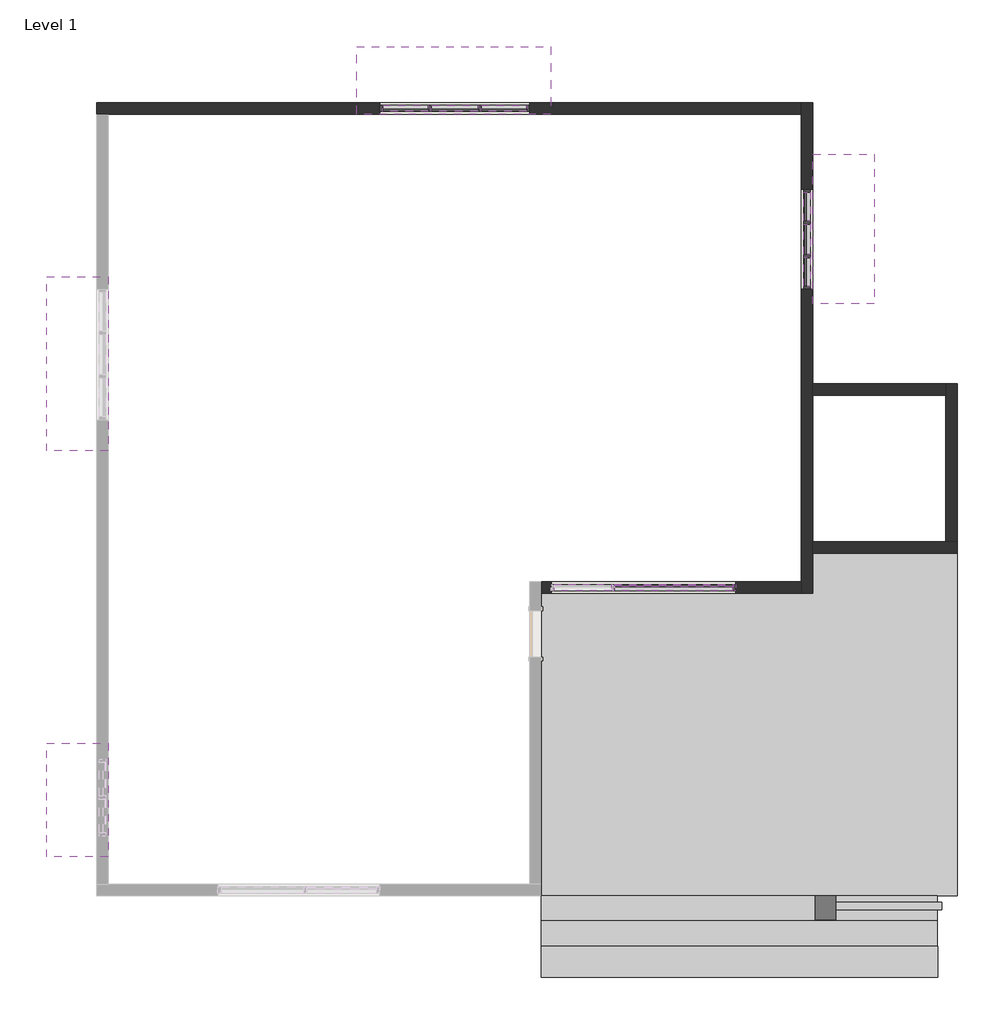
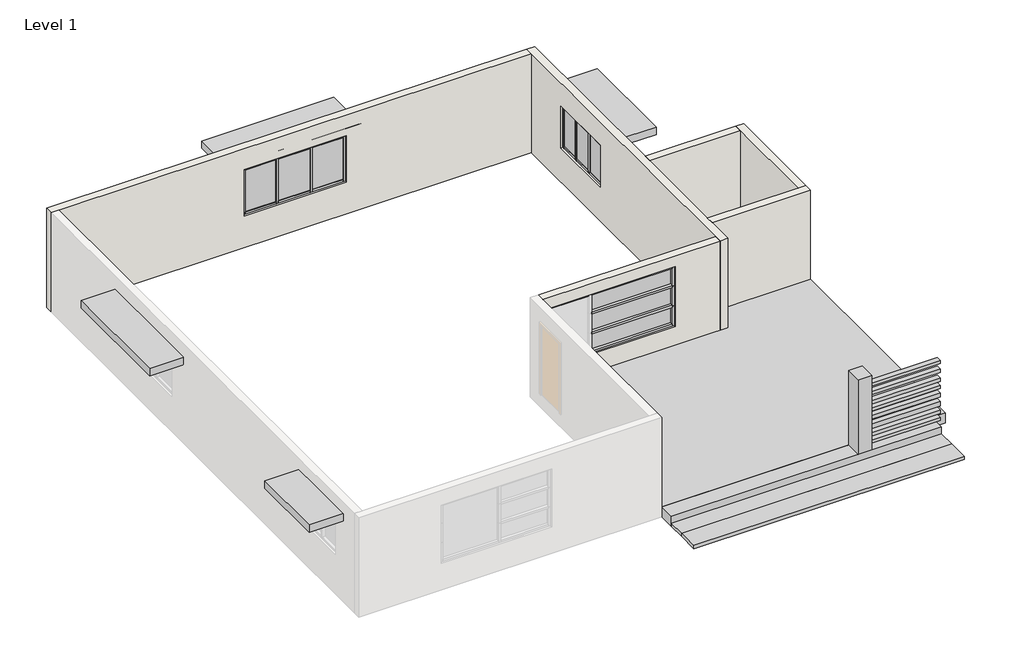
# One storey, part 2 of 2: 28 members, 9 plates, 6 proxies, 6 walls.
"""IFC4 building model written with IfcOpenShell, lengths in millimetres."""

from ifc_helpers import new_model, si_unit, frame, origin, origin_with_axes, place, context, project, spatial, polyline, outline, extrude, faceted_brep, transform, mapped, element, save
from components import generic_models_1_generic_models_1_8617edb6, generic_models_4_generic_models_4_7ae05182, generic_models_5_generic_models_5_11858d31, generic_models_6_generic_models_6_1132ce1b, generic_models_7_generic_models_7_82613ab6, generic_models_8_generic_models_8_38ca69cf, member_e6b9f524, member_eadc486f, member_9597caa3, member_b864958b, member_a400357f, member_6f432376, member_b9a8557f, member_093c7ff9, member_f1f71bde, member_f689fba6, member_6283365f, member_80b92b34, system_panel_glazed_646da070, system_panel_glazed_ba5e2c5f, system_panel_glazed_ed2f53c1, system_panel_glazed_6a84950c, system_panel_glazed_e669d95e, system_panel_glazed_5df0e43d

model = new_model("IFC4")

# Units and contexts
model_context = context("Model", 3, world=origin())
ifc_project = project(units=[si_unit("LENGTHUNIT", "METRE", prefix="MILLI")], contexts=[model_context])

# Site, building, storey
site = spatial("IfcSite", under=ifc_project)
building = spatial("IfcBuilding", under=site)
storey = spatial("IfcBuildingStorey", under=building, Name="Level 1", Elevation=0.0)

# Proxies
placement = place(None, origin())
generic_models_1_generic_models_1_shape = generic_models_1_generic_models_1_8617edb6(model_context)
element("IfcBuildingElementProxy", 1, Name="Generic Models 1 : Generic Models 1", ObjectType="Generic Models 1 : Generic Models 1", at=placement, inside=storey, context=model_context, shape_type="MappedRepresentation", body=[
    mapped(generic_models_1_generic_models_1_shape, transform((0.0, 0.0, 0.0), x_axis=(1.0, 0.0, 0.0), y_axis=(0.0, 1.0, 0.0), z_axis=(0.0, 0.0, 1.0))),
])
generic_models_4_generic_models_4_shape = generic_models_4_generic_models_4_7ae05182(model_context)
element("IfcBuildingElementProxy", 2, Name="Generic Models 4 : Generic Models 4", ObjectType="Generic Models 4 : Generic Models 4", at=placement, inside=storey, context=model_context, shape_type="MappedRepresentation", body=[
    mapped(generic_models_4_generic_models_4_shape, transform((0.0, 0.0, 0.0), x_axis=(1.0, 0.0, 0.0), y_axis=(0.0, 1.0, 0.0), z_axis=(0.0, 0.0, 1.0))),
])
generic_models_5_generic_models_5_shape = generic_models_5_generic_models_5_11858d31(model_context)
element("IfcBuildingElementProxy", 3, Name="Generic Models 5 : Generic Models 5", ObjectType="Generic Models 5 : Generic Models 5", at=placement, inside=storey, context=model_context, shape_type="MappedRepresentation", body=[
    mapped(generic_models_5_generic_models_5_shape, transform((0.0, 0.0, 0.0), x_axis=(1.0, 0.0, 0.0), y_axis=(0.0, 1.0, 0.0), z_axis=(0.0, 0.0, 1.0))),
])
generic_models_6_generic_models_6_shape = generic_models_6_generic_models_6_1132ce1b(model_context)
element("IfcBuildingElementProxy", 4, Name="Generic Models 6 : Generic Models 6", ObjectType="Generic Models 6 : Generic Models 6", at=placement, inside=storey, context=model_context, shape_type="MappedRepresentation", body=[
    mapped(generic_models_6_generic_models_6_shape, transform((0.0, 0.0, 0.0), x_axis=(1.0, 0.0, 0.0), y_axis=(0.0, 1.0, 0.0), z_axis=(0.0, 0.0, 1.0))),
])
generic_models_7_generic_models_7_shape = generic_models_7_generic_models_7_82613ab6(model_context)
element("IfcBuildingElementProxy", 5, Name="Generic Models 7 : Generic Models 7", ObjectType="Generic Models 7 : Generic Models 7", at=placement, inside=storey, context=model_context, shape_type="MappedRepresentation", body=[
    mapped(generic_models_7_generic_models_7_shape, transform((0.0, 0.0, 0.0), x_axis=(1.0, 0.0, 0.0), y_axis=(0.0, 1.0, 0.0), z_axis=(0.0, 0.0, 1.0))),
])
generic_models_8_generic_models_8_shape = generic_models_8_generic_models_8_38ca69cf(model_context)
element("IfcBuildingElementProxy", 6, Name="Generic Models 8 : Generic Models 8", ObjectType="Generic Models 8 : Generic Models 8", at=placement, inside=storey, context=model_context, shape_type="MappedRepresentation", body=[
    mapped(generic_models_8_generic_models_8_shape, transform((0.0, 0.0, 0.0), x_axis=(1.0, 0.0, 0.0), y_axis=(0.0, 1.0, 0.0), z_axis=(0.0, 0.0, 1.0))),
])

# Members
member_shape = member_e6b9f524(model_context)
element("IfcMember", 7, ObjectType="Rectangular Mullion : 2.5\" x 5\" rectangular", at=placement, inside=storey, context=model_context, shape_type="MappedRepresentation", body=[
    mapped(member_shape, transform((-9865.5620831, -6017.2945627, 2710.3034891), x_axis=(0.0, 0.0, 1.0), y_axis=(0.0, -1.0, 0.0), z_axis=(1.0, 0.0, 0.0))),
])
member_2_shape = member_eadc486f(model_context)
element("IfcMember", 8, ObjectType="Rectangular Mullion : 2.5\" x 5\" rectangular", at=placement, inside=storey, context=model_context, shape_type="MappedRepresentation", body=[
    mapped(member_2_shape, transform((-7458.9120831, -6017.2945627, 2710.3034891), x_axis=(0.0, 0.0, 1.0), y_axis=(0.0, -1.0, 0.0), z_axis=(1.0, 0.0, 0.0))),
])
element("IfcMember", 9, ObjectType="Rectangular Mullion : 2.5\" x 5\" rectangular", at=placement, inside=storey, context=model_context, shape_type="MappedRepresentation", body=[
    mapped(member_2_shape, transform((-9802.0620831, -6017.2945627, 871.9220892), x_axis=(0.0, 0.0, -1.0), y_axis=(0.0, -1.0, 0.0), z_axis=(-1.0, 0.0, 0.0))),
])
member_3_shape = member_9597caa3(model_context)
element("IfcMember", 10, ObjectType="Rectangular Mullion : 2.5\" x 5\" rectangular", at=placement, inside=storey, context=model_context, shape_type="MappedRepresentation", body=[
    mapped(member_3_shape, transform((-7458.9120831, -6017.2945627, 2097.5096891), x_axis=(0.0, 0.0, 1.0), y_axis=(0.0, -1.0, 0.0), z_axis=(1.0, 0.0, 0.0))),
])
element("IfcMember", 11, ObjectType="Rectangular Mullion : 2.5\" x 5\" rectangular", at=placement, inside=storey, context=model_context, shape_type="MappedRepresentation", body=[
    mapped(member_3_shape, transform((-7458.9120831, -6017.2945627, 1484.7158892), x_axis=(0.0, 0.0, 1.0), y_axis=(0.0, -1.0, 0.0), z_axis=(1.0, 0.0, 0.0))),
])
member_4_shape = member_b864958b(model_context)
element("IfcMember", 12, ObjectType="Rectangular Mullion : 2.5\" x 5\" rectangular", at=placement, inside=storey, context=model_context, shape_type="MappedRepresentation", body=[
    mapped(member_4_shape, transform((-7395.4120831, -6017.2945627, 1484.7158892), x_axis=(1.0, 0.0, 0.0), y_axis=(0.0, -1.0, 0.0), z_axis=(0.0, 0.0, -1.0))),
])
element("IfcMember", 13, ObjectType="Rectangular Mullion : 2.5\" x 5\" rectangular", at=placement, inside=storey, context=model_context, shape_type="MappedRepresentation", body=[
    mapped(member_4_shape, transform((-7395.4120831, -6017.2945627, 2097.5096891), x_axis=(1.0, 0.0, 0.0), y_axis=(0.0, -1.0, 0.0), z_axis=(0.0, 0.0, -1.0))),
])
element("IfcMember", 14, ObjectType="Rectangular Mullion : 2.5\" x 5\" rectangular", at=placement, inside=storey, context=model_context, shape_type="MappedRepresentation", body=[
    mapped(member_4_shape, transform((-7395.4120831, -6017.2945627, 871.9220892), x_axis=(1.0, 0.0, 0.0), y_axis=(0.0, -1.0, 0.0), z_axis=(0.0, 0.0, -1.0))),
])
member_5_shape = member_a400357f(model_context)
element("IfcMember", 15, ObjectType="Rectangular Mullion : 2.5\" x 5\" rectangular", at=placement, inside=storey, context=model_context, shape_type="MappedRepresentation", body=[
    mapped(member_5_shape, transform((-5985.7120831, 1177.2554373, 2338.9510739), x_axis=(0.0, 0.0, 1.0), y_axis=(1.0, 0.0, 0.0), z_axis=(0.0, 1.0, 0.0))),
])
member_6_shape = member_6f432376(model_context)
element("IfcMember", 16, ObjectType="Rectangular Mullion : 2.5\" x 5\" rectangular", at=placement, inside=storey, context=model_context, shape_type="MappedRepresentation", body=[
    mapped(member_6_shape, transform((-5985.7120831, 516.8554373, 2338.9510739), x_axis=(0.0, 0.0, 1.0), y_axis=(1.0, 0.0, 0.0), z_axis=(0.0, 1.0, 0.0))),
])
element("IfcMember", 17, ObjectType="Rectangular Mullion : 2.5\" x 5\" rectangular", at=placement, inside=storey, context=model_context, shape_type="MappedRepresentation", body=[
    mapped(member_6_shape, transform((-5985.7120831, 1805.9054373, 2338.9510739), x_axis=(0.0, 0.0, 1.0), y_axis=(1.0, 0.0, 0.0), z_axis=(0.0, 1.0, 0.0))),
])
member_7_shape = member_b9a8557f(model_context)
element("IfcMember", 18, ObjectType="Rectangular Mullion : 2.5\" x 5\" rectangular", at=placement, inside=storey, context=model_context, shape_type="MappedRepresentation", body=[
    mapped(member_7_shape, transform((-5985.7120831, 548.6054373, 1049.9895234), x_axis=(0.0, 1.0, 0.0), y_axis=(1.0, 0.0, 0.0), z_axis=(0.0, 0.0, -1.0))),
])
element("IfcMember", 19, ObjectType="Rectangular Mullion : 2.5\" x 5\" rectangular", at=placement, inside=storey, context=model_context, shape_type="MappedRepresentation", body=[
    mapped(member_7_shape, transform((-5985.7120831, 1209.0054373, 1049.9895234), x_axis=(0.0, 1.0, 0.0), y_axis=(1.0, 0.0, 0.0), z_axis=(0.0, 0.0, -1.0))),
])
element("IfcMember", 20, ObjectType="Rectangular Mullion : 2.5\" x 5\" rectangular", at=placement, inside=storey, context=model_context, shape_type="MappedRepresentation", body=[
    mapped(member_5_shape, transform((-5985.7120831, 580.3554373, 1049.9895234), x_axis=(0.0, 0.0, -1.0), y_axis=(1.0, 0.0, 0.0), z_axis=(0.0, -1.0, 0.0))),
])
element("IfcMember", 21, ObjectType="Rectangular Mullion : 2.5\" x 5\" rectangular", at=placement, inside=storey, context=model_context, shape_type="MappedRepresentation", body=[
    mapped(member_6_shape, transform((-5985.7120831, 1240.7554373, 1049.9895234), x_axis=(0.0, 0.0, -1.0), y_axis=(1.0, 0.0, 0.0), z_axis=(0.0, -1.0, 0.0))),
])
element("IfcMember", 22, ObjectType="Rectangular Mullion : 2.5\" x 5\" rectangular", at=placement, inside=storey, context=model_context, shape_type="MappedRepresentation", body=[
    mapped(member_6_shape, transform((-5985.7120831, -48.2945627, 1049.9895234), x_axis=(0.0, 0.0, -1.0), y_axis=(1.0, 0.0, 0.0), z_axis=(0.0, -1.0, 0.0))),
])
member_8_shape = member_093c7ff9(model_context)
element("IfcMember", 23, ObjectType="Rectangular Mullion : 2.5\" x 5\" rectangular", at=placement, inside=storey, context=model_context, shape_type="MappedRepresentation", body=[
    mapped(member_8_shape, transform((-5985.7120831, -111.7945627, 2338.9510739), x_axis=(0.0, -1.0, 0.0), y_axis=(1.0, 0.0, 0.0), z_axis=(0.0, 0.0, 1.0))),
])
element("IfcMember", 24, ObjectType="Rectangular Mullion : 2.5\" x 5\" rectangular", at=placement, inside=storey, context=model_context, shape_type="MappedRepresentation", body=[
    mapped(member_8_shape, transform((-5985.7120831, 1869.4054373, 1049.9895234), x_axis=(0.0, 1.0, 0.0), y_axis=(1.0, 0.0, 0.0), z_axis=(0.0, 0.0, -1.0))),
])
member_9_shape = member_f1f71bde(model_context)
element("IfcMember", 25, ObjectType="Rectangular Mullion : 2.5\" x 5\" rectangular", at=placement, inside=storey, context=model_context, shape_type="MappedRepresentation", body=[
    mapped(member_9_shape, transform((-12430.9620831, 3469.6054373, 2408.3377855), x_axis=(0.0, 0.0, 1.0), y_axis=(0.0, 1.0, 0.0), z_axis=(-1.0, 0.0, 0.0))),
])
element("IfcMember", 26, ObjectType="Rectangular Mullion : 2.5\" x 5\" rectangular", at=placement, inside=storey, context=model_context, shape_type="MappedRepresentation", body=[
    mapped(member_9_shape, transform((-14380.4120831, 3469.6054373, 2408.3377855), x_axis=(0.0, 0.0, 1.0), y_axis=(0.0, 1.0, 0.0), z_axis=(-1.0, 0.0, 0.0))),
])
member_10_shape = member_f689fba6(model_context)
element("IfcMember", 27, ObjectType="Rectangular Mullion : 2.5\" x 5\" rectangular", at=placement, inside=storey, context=model_context, shape_type="MappedRepresentation", body=[
    mapped(member_10_shape, transform((-13421.5620831, 3469.6054373, 2408.3377855), x_axis=(0.0, 0.0, 1.0), y_axis=(0.0, 1.0, 0.0), z_axis=(-1.0, 0.0, 0.0))),
])
member_11_shape = member_6283365f(model_context)
element("IfcMember", 28, ObjectType="Rectangular Mullion : 2.5\" x 5\" rectangular", at=placement, inside=storey, context=model_context, shape_type="MappedRepresentation", body=[
    mapped(member_11_shape, transform((-12462.7120831, 3469.6054373, 986.2085001), x_axis=(-1.0, 0.0, 0.0), y_axis=(0.0, 1.0, 0.0), z_axis=(0.0, 0.0, -1.0))),
])
element("IfcMember", 29, ObjectType="Rectangular Mullion : 2.5\" x 5\" rectangular", at=placement, inside=storey, context=model_context, shape_type="MappedRepresentation", body=[
    mapped(member_11_shape, transform((-13453.3120831, 3469.6054373, 986.2085001), x_axis=(-1.0, 0.0, 0.0), y_axis=(0.0, 1.0, 0.0), z_axis=(0.0, 0.0, -1.0))),
])
element("IfcMember", 30, ObjectType="Rectangular Mullion : 2.5\" x 5\" rectangular", at=placement, inside=storey, context=model_context, shape_type="MappedRepresentation", body=[
    mapped(member_9_shape, transform((-13485.0620831, 3469.6054373, 986.2085001), x_axis=(0.0, 0.0, -1.0), y_axis=(0.0, 1.0, 0.0), z_axis=(1.0, 0.0, 0.0))),
])
element("IfcMember", 31, ObjectType="Rectangular Mullion : 2.5\" x 5\" rectangular", at=placement, inside=storey, context=model_context, shape_type="MappedRepresentation", body=[
    mapped(member_9_shape, transform((-11535.6120831, 3469.6054373, 986.2085001), x_axis=(0.0, 0.0, -1.0), y_axis=(0.0, 1.0, 0.0), z_axis=(1.0, 0.0, 0.0))),
])
element("IfcMember", 32, ObjectType="Rectangular Mullion : 2.5\" x 5\" rectangular", at=placement, inside=storey, context=model_context, shape_type="MappedRepresentation", body=[
    mapped(member_10_shape, transform((-12494.4620831, 3469.6054373, 986.2085001), x_axis=(0.0, 0.0, -1.0), y_axis=(0.0, 1.0, 0.0), z_axis=(1.0, 0.0, 0.0))),
])
member_12_shape = member_80b92b34(model_context)
element("IfcMember", 33, ObjectType="Rectangular Mullion : 2.5\" x 5\" rectangular", at=placement, inside=storey, context=model_context, shape_type="MappedRepresentation", body=[
    mapped(member_12_shape, transform((-11472.1120831, 3469.6054373, 2408.3377855), x_axis=(1.0, 0.0, 0.0), y_axis=(0.0, 1.0, 0.0), z_axis=(0.0, 0.0, 1.0))),
])
element("IfcMember", 34, ObjectType="Rectangular Mullion : 2.5\" x 5\" rectangular", at=placement, inside=storey, context=model_context, shape_type="MappedRepresentation", body=[
    mapped(member_12_shape, transform((-14443.9120831, 3469.6054373, 986.2085001), x_axis=(-1.0, 0.0, 0.0), y_axis=(0.0, 1.0, 0.0), z_axis=(0.0, 0.0, -1.0))),
])

# Plates
system_panel_glazed_shape = system_panel_glazed_646da070(model_context)
element("IfcPlate", 35, ObjectType="System Panel : Glazed", at=placement, inside=storey, context=model_context, shape_type="MappedRepresentation", body=[
    mapped(system_panel_glazed_shape, transform((-8630.4870831, -6017.2945627, 935.4220892), x_axis=(1.0, 0.0, 0.0), y_axis=(0.0, 1.0, 0.0), z_axis=(0.0, 0.0, 1.0))),
])
element("IfcPlate", 36, ObjectType="System Panel : Glazed", at=placement, inside=storey, context=model_context, shape_type="MappedRepresentation", body=[
    mapped(system_panel_glazed_shape, transform((-8630.4870831, -6017.2945627, 2129.2596891), x_axis=(1.0, 0.0, 0.0), y_axis=(0.0, 1.0, 0.0), z_axis=(0.0, 0.0, 1.0))),
])
system_panel_glazed_2_shape = system_panel_glazed_ba5e2c5f(model_context)
element("IfcPlate", 37, ObjectType="System Panel : Glazed", at=placement, inside=storey, context=model_context, shape_type="MappedRepresentation", body=[
    mapped(system_panel_glazed_2_shape, transform((-8630.4870831, -6017.2945627, 1516.4658892), x_axis=(1.0, 0.0, 0.0), y_axis=(0.0, 1.0, 0.0), z_axis=(0.0, 0.0, 1.0))),
])
system_panel_glazed_3_shape = system_panel_glazed_ed2f53c1(model_context)
element("IfcPlate", 38, ObjectType="System Panel : Glazed", at=placement, inside=storey, context=model_context, shape_type="MappedRepresentation", body=[
    mapped(system_panel_glazed_3_shape, transform((-5985.7120831, 234.2804373, 1113.4895234), x_axis=(0.0, 1.0, 0.0), y_axis=(-1.0, 0.0, 0.0), z_axis=(0.0, 0.0, 1.0))),
])
element("IfcPlate", 39, ObjectType="System Panel : Glazed", at=placement, inside=storey, context=model_context, shape_type="MappedRepresentation", body=[
    mapped(system_panel_glazed_3_shape, transform((-5985.7120831, 1523.3304373, 1113.4895234), x_axis=(0.0, 1.0, 0.0), y_axis=(-1.0, 0.0, 0.0), z_axis=(0.0, 0.0, 1.0))),
])
system_panel_glazed_4_shape = system_panel_glazed_6a84950c(model_context)
element("IfcPlate", 40, ObjectType="System Panel : Glazed", at=placement, inside=storey, context=model_context, shape_type="MappedRepresentation", body=[
    mapped(system_panel_glazed_4_shape, transform((-5985.7120831, 878.8054373, 1113.4895234), x_axis=(0.0, 1.0, 0.0), y_axis=(-1.0, 0.0, 0.0), z_axis=(0.0, 0.0, 1.0))),
])
system_panel_glazed_5_shape = system_panel_glazed_e669d95e(model_context)
element("IfcPlate", 41, ObjectType="System Panel : Glazed", at=placement, inside=storey, context=model_context, shape_type="MappedRepresentation", body=[
    mapped(system_panel_glazed_5_shape, transform((-11983.2870831, 3469.6054373, 1049.7085001), x_axis=(-1.0, 0.0, 0.0), y_axis=(0.0, -1.0, 0.0), z_axis=(0.0, 0.0, 1.0))),
])
element("IfcPlate", 42, ObjectType="System Panel : Glazed", at=placement, inside=storey, context=model_context, shape_type="MappedRepresentation", body=[
    mapped(system_panel_glazed_5_shape, transform((-13932.7370831, 3469.6054373, 1049.7085001), x_axis=(-1.0, 0.0, 0.0), y_axis=(0.0, -1.0, 0.0), z_axis=(0.0, 0.0, 1.0))),
])
system_panel_glazed_6_shape = system_panel_glazed_5df0e43d(model_context)
element("IfcPlate", 43, ObjectType="System Panel : Glazed", at=placement, inside=storey, context=model_context, shape_type="MappedRepresentation", body=[
    mapped(system_panel_glazed_6_shape, transform((-12958.0120831, 3469.6054373, 1049.7085001), x_axis=(-1.0, 0.0, 0.0), y_axis=(0.0, -1.0, 0.0), z_axis=(0.0, 0.0, 1.0))),
])

# Walls
element("IfcWall", 44, ObjectType="9\"", at=placement, inside=storey, context=model_context, shape_type="Brep", body=[
    faceted_brep([(-6100.0120831, 3583.9054373, 0.0), (-20044.6120831, 3583.9054373, 0.0), (-20044.6120831, 3583.9054373, 3048.0), (-6100.0120831, 3583.9054373, 3048.0), (-11472.1120831, 3583.9054373, 986.2085001), (-11472.1120831, 3583.9054373, 2408.3377855), (-14443.9120831, 3583.9054373, 2408.3377855), (-14443.9120831, 3583.9054373, 986.2085001), (-20044.6120831, 3355.3054373, 0.0), (-19816.0120831, 3355.3054373, 0.0), (-6100.0120831, 3355.3054373, 0.0), (-6100.0120831, 3355.3054373, 3048.0), (-19816.0120831, 3355.3054373, 3048.0), (-20044.6120831, 3355.3054373, 3048.0), (-11472.1120831, 3355.3054373, 2408.3377855), (-11472.1120831, 3355.3054373, 986.2085001), (-14443.9120831, 3355.3054373, 986.2085001), (-14443.9120831, 3355.3054373, 2408.3377855)], [[[0, 1, 2, 3], [4, 5, 6, 7]], [[8, 9, 10, 11, 12, 13], [14, 15, 16, 17]], [[1, 0, 10, 9, 8]], [[3, 2, 13, 12, 11]], [[0, 3, 11, 10]], [[2, 1, 8, 13]], [[4, 15, 14, 5]], [[5, 14, 17, 6]], [[6, 17, 16, 7]], [[15, 4, 7, 16]]]),
])
element("IfcWall", 45, ObjectType="9\"", at=placement, inside=storey, context=model_context, shape_type="SweptSolid", body=[
    extrude(outline(polyline([(0.0, -11243.5120831), (0.0, -6100.0120831), (3048.0, -6100.0120831), (3048.0, -11243.5120831), (0.0, -11243.5120831)]), holes=[polyline([(871.9220892, -11053.0120831), (2710.3034891, -11053.0120831), (2710.3034891, -7395.4120831), (871.9220892, -7395.4120831), (871.9220892, -11053.0120831)])]), frame((0.0, -6131.5945627, 0.0), z_axis=(0.0, 1.0, 0.0), x_axis=(0.0, 0.0, 1.0)), (0.0, 0.0, 1.0), 228.6),
])
element("IfcWall", 46, ObjectType="9\"", at=placement, inside=storey, context=model_context, shape_type="Brep", body=[
    faceted_brep([(-5871.4120831, -5331.4945627, 0.0), (-3013.9120831, -5331.4945627, 0.0), (-3013.9120831, -5331.4945627, 3048.0), (-5871.4120831, -5331.4945627, 3048.0), (-5871.4120831, -5102.8945627, 0.0), (-5871.4120831, -5102.8945627, 3048.0), (-3242.5120831, -5102.8945627, 3048.0), (-3013.9120831, -5102.8945627, 3048.0), (-3013.9120831, -5102.8945627, 0.0), (-3242.5120831, -5102.8945627, 0.0)], [[[0, 1, 2, 3]], [[4, 5, 6, 7, 8, 9]], [[1, 0, 4, 9, 8]], [[3, 2, 7, 6, 5]], [[0, 3, 5, 4]], [[2, 1, 8, 7]]]),
])
element("IfcWall", 47, ObjectType="9\"", at=placement, inside=storey, context=model_context, shape_type="Brep", body=[
    faceted_brep([(-3013.9120831, -5102.8945627, 0.0), (-3013.9120831, -1978.6945627, 0.0), (-3013.9120831, -1978.6945627, 3048.0), (-3013.9120831, -5102.8945627, 3048.0), (-3242.5120831, -5102.8945627, 0.0), (-3242.5120831, -5102.8945627, 3048.0), (-3242.5120831, -2207.2945627, 3048.0), (-3242.5120831, -1978.6945627, 3048.0), (-3242.5120831, -1978.6945627, 0.0), (-3242.5120831, -2207.2945627, 0.0)], [[[0, 1, 2, 3]], [[4, 5, 6, 7, 8, 9]], [[1, 0, 4, 9, 8]], [[3, 2, 7, 6, 5]], [[0, 3, 5, 4]], [[2, 1, 8, 7]]]),
])
element("IfcWall", 48, ObjectType="9\"", at=placement, inside=storey, context=model_context, shape_type="SweptSolid", body=[
    extrude(outline(polyline([(-5871.4120831, -1978.6945627), (-3242.5120831, -1978.6945627), (-3242.5120831, -2207.2945627), (-5871.4120831, -2207.2945627), (-5871.4120831, -1978.6945627)])), origin_with_axes(), (0.0, 0.0, 1.0), 3048.0),
])
element("IfcWall", 49, ObjectType="9\"", at=placement, inside=storey, context=model_context, shape_type="Brep", body=[
    faceted_brep([(-5871.4120831, -6131.5945627, 0.0), (-5871.4120831, -5331.4945627, 0.0), (-5871.4120831, -5102.8945627, 0.0), (-5871.4120831, -2207.2945627, 0.0), (-5871.4120831, -1978.6945627, 0.0), (-5871.4120831, 3583.9054373, 0.0), (-5871.4120831, 3583.9054373, 3048.0), (-5871.4120831, -1978.6945627, 3048.0), (-5871.4120831, -2207.2945627, 3048.0), (-5871.4120831, -5102.8945627, 3048.0), (-5871.4120831, -5331.4945627, 3048.0), (-5871.4120831, -6131.5945627, 3048.0), (-5871.4120831, -111.7945627, 1049.9895234), (-5871.4120831, -111.7945627, 2338.9510739), (-5871.4120831, 1869.4054373, 2338.9510739), (-5871.4120831, 1869.4054373, 1049.9895234), (-6100.0120831, 3583.9054373, 0.0), (-6100.0120831, 3355.3054373, 0.0), (-6100.0120831, -5902.9945627, 0.0), (-6100.0120831, -6131.5945627, 0.0), (-6100.0120831, -6131.5945627, 3048.0), (-6100.0120831, -5902.9945627, 3048.0), (-6100.0120831, 3355.3054373, 3048.0), (-6100.0120831, 3583.9054373, 3048.0), (-6100.0120831, -111.7945627, 2338.9510739), (-6100.0120831, -111.7945627, 1049.9895234), (-6100.0120831, 1869.4054373, 1049.9895234), (-6100.0120831, 1869.4054373, 2338.9510739)], [[[0, 1, 2, 3, 4, 5, 6, 7, 8, 9, 10, 11], [12, 13, 14, 15]], [[16, 17, 18, 19, 20, 21, 22, 23], [24, 25, 26, 27]], [[5, 4, 3, 2, 1, 0, 19, 18, 17, 16]], [[11, 10, 9, 8, 7, 6, 23, 22, 21, 20]], [[0, 11, 20, 19]], [[6, 5, 16, 23]], [[12, 25, 24, 13]], [[13, 24, 27, 14]], [[14, 27, 26, 15]], [[25, 12, 15, 26]]]),
])

save(model, "model.ifc")

# Revit data of these elements
# Type "Rectangular Mullion : 2.5\" x 5\" rectangular"
#   built-in parameter 1007304 = 0.416667 (stored number, unit not read)
#   built-in parameter 1007301 = 0.104167 (stored number, unit not read)
#   built-in parameter 1007300 = 0.104167 (stored number, unit not read)
# Type "System Panel : Glazed"
#   Construction Type Id = "GSP4R"
#   Analytic Construction = "1/8 in Pilkington single glazing"
#   Visual Light Transmittance = 0.9
#   Solar Heat Gain Coefficient = 0.86
#   Heat Transfer Coefficient (U) = 1.18115 BTU/(h·ft²·°F)
#   Define Thermal Properties by = 1
# Type "9\""
#   Assembly Code = "B2010"
#   Layers, outside or top first: 0' - 9" no material (function 1)
# Element 1 (IfcBuildingElementProxy, "Generic Models 1 : Generic Models 1")
#   Phase Created = New Construction
# Element 2 (IfcBuildingElementProxy, "Generic Models 4 : Generic Models 4")
#   Phase Created = New Construction
# Element 3 (IfcBuildingElementProxy, "Generic Models 5 : Generic Models 5")
#   Phase Created = New Construction
# Element 4 (IfcBuildingElementProxy, "Generic Models 6 : Generic Models 6")
#   Phase Created = New Construction
# Element 5 (IfcBuildingElementProxy, "Generic Models 7 : Generic Models 7")
#   Phase Created = New Construction
# Element 6 (IfcBuildingElementProxy, "Generic Models 8 : Generic Models 8")
#   Phase Created = New Construction
# Elements 7, 8, 9, 10, 11, 12, 13, 14, 15, 16, 17, 18, 19, 20, 21, 22, 23, 24, 25, 26, 27, 28, 29, 30, 31, 32, 33, 34 (IfcMember, "Rectangular Mullion : 2.5\" x 5\" rectangular")
#   Phase Created = New Construction
#   Materials on its faces: "Aluminum"
# Elements 35, 36, 37, 38, 39, 40, 41, 42, 43 (IfcPlate, "System Panel : Glazed")
#   Phase Created = New Construction
#   Materials on its faces: "Glass"
# Elements 44, 45, 46, 47, 48, 49 (IfcWall, "9\"")
#   Top Offset = 0' - 0"
#   Base Offset = 0' - 0"
#   Unconnected Height = 10' - 0"
#   wall height = 10' - 0"
#   Phase Created = New Construction
#   Base Constraint = Level 1
#   Materials on its faces: "Default Wall"
# Materials
#   "Aluminum": class "Metal", colour RGB 247 247 247, transparency 0, Description = "Aluminum 6061", Cost = 0
#   "Glass": class "Glass", colour RGB 0 128 192, transparency 0.75, Description = "Soda Lime Glass", Cost = 0
#   "Default Wall": colour RGB 128 128 128, transparency 0, Cost = 0
